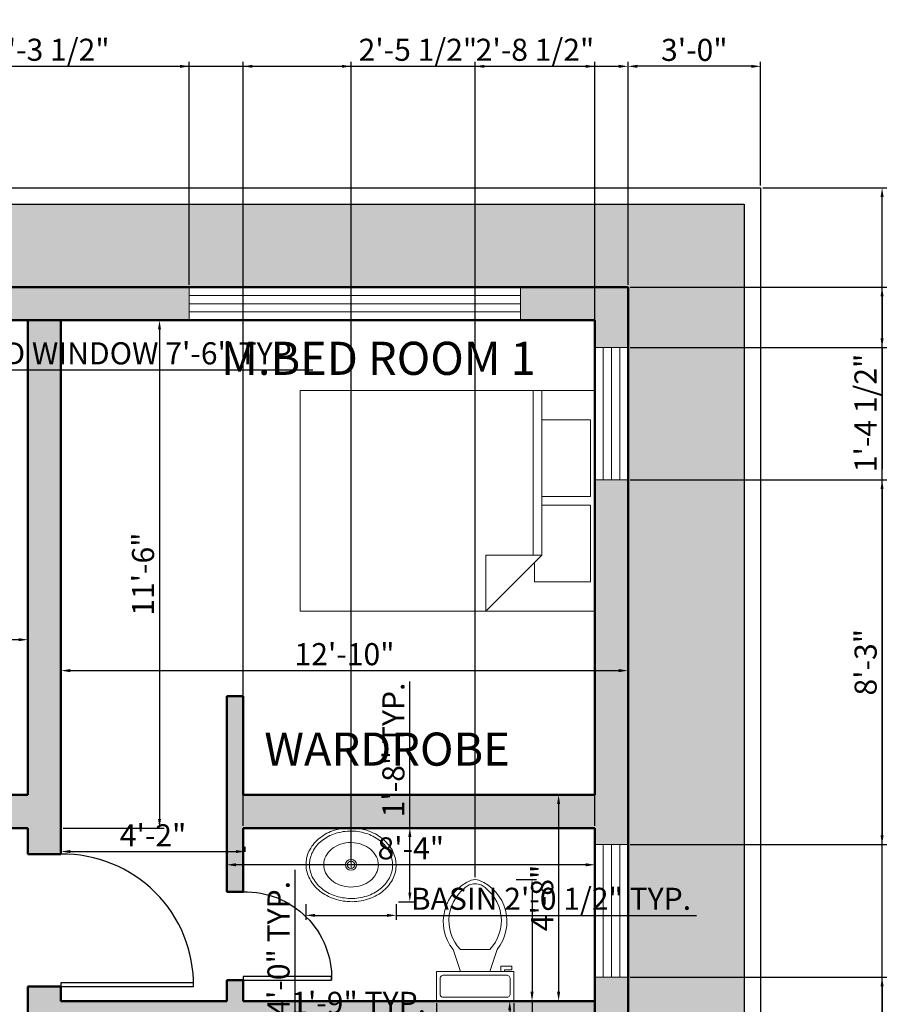
# Model space of a CAD drawing. Units: inches. Extents: x 2623 to 3157, y 1514 to 2273.
# Tile 6 of 6: x 2917 to 3157, y 1991 to 2258. Entities that reach past the tile are written whole.
import ezdxf

# ---------------------------------------------------------------- set-up
doc = ezdxf.new("R2010")
doc.units = ezdxf.units.IN
for name, color, linetype, lineweight in [('A-ANNO-DIMS', 2, 'Continuous', 18), ('A-AREA-IDEN', 7, 'Continuous', 25), ('A-DOOR', 4, 'Continuous', 25), ('A-FLOR-FIXT', 9, 'Continuous', 18), ('A-FURN', 8, 'Continuous', 18), ('A-GLAZ', 4, 'Continuous', 20), ('A-WALL', 7, 'Continuous', 50), ('A-WALL-PATT', 252, 'Continuous', 13), ('C-PROP', 7, 'Continuous', 25), ('L-PLNT-PATT', 9, 'Continuous', 13)]:
    doc.layers.add(name, color=color, linetype=linetype, lineweight=lineweight)
doc.styles.get("Standard").update_dxf_attribs({"font": 'arial.ttf'})
doc.dimstyles.new('ISO-25', dxfattribs={"dimtxt": 6, "dimasz": 2.5, "dimexe": 1.25, "dimexo": 0.625, "dimtad": 1, "dimdec": 1, "dimlunit": 3, "dimtxsty": 'Standard', "dimcen": 2.5, "dimadec": 0, "dimazin": 0, "dimtfac": 1, "dimtdec": 1, "dimtmove": 0, "dimatfit": 3, "dimfxl": 1, "dimarcsym": 0})

# ---------------------------------------------------------------- blocks, each defined once
blk = doc.blocks.new('Toilet - top')
for p, q in [((9.5, -6), (9.5, -2)), ((-8, -8.5), (-8, -8)), ((-7, -8), (-7, -9.5)), ((-4, -8), (-6, -14)), ((4, -8), (6, -14)), ((-10, -8.5), (-8, -8.5)), ((-10, -9.5), (-10, -8.5)), ((-7, -9.5), (-10, -9.5)), ((4, -14), (-4, -14))]:
    blk.add_line(p, q)
blk.add_lwpolyline([(10.5, -8), (10.5, 0), (-10.5, 0), (-10.5, -8)], close=True)
for points in [[(-9.5, -2), (-9.5, -6)], [(8.5, -1), (-8.5, -1)], [(-8.5, -7), (8.5, -7)]]:
    blk.add_lwpolyline(points)
for centre, radius, start, end in [((-8.62, -1.88), 0.884, 81.8699, 188.1301), ((8.62, -1.88), 0.884, 351.8699, 98.1301), ((-8.62, -6.12), 0.884, 171.8699, 278.1301), ((8.62, -6.12), 0.884, 261.8699, 8.1301), ((3.52, -21.58), 12.17, 141.4691, 247.9714), ((4.2, -21.82), 11.33, 136.3677, 238.9468), ((-3.52, -21.58), 12.17, 292.0284, 38.5307), ((-4.2, -21.82), 11.33, 301.053, 43.6321), ((0, -27.88), 4, 245.7318, 294.2682), ((0, -29), 4, 254.8605, 285.1395)]:
    blk.add_arc(centre, radius, start, end)
blk = doc.blocks.new('Sink - Oval top')
for p, q in [((-1, 0), (1, 0)), ((0, 1), (0, -1))]:
    blk.add_line(p, q)
for points in [[(-12.23, 0.39, 0.117634), (-11.46, -3.36, 0.104469), (-8.88, -6.8, 0.090016), (-5.08, -9.07, 0.08192), (-0.32, -10.02, 0.08192), (4.49, -9.38, 0.090016), (8.42, -7.36, 0.104469), (11.22, -4.09, 0.117634), (12.23, -0.39, 0.117634), (11.46, 3.36, 0.104469), (8.88, 6.8, 0.090016), (5.08, 9.07, 0.08192), (0.32, 10.02, 0.08192), (-4.49, 9.38, 0.090016), (-8.42, 7.36, 0.104469), (-11.22, 4.09, 0.117634)], [(-11.29, 0.16, 0.118622), (-10.52, -3.25, 0.104678), (-8.07, -6.36, 0.089562), (-4.54, -8.37, 0.081185), (-0.13, -9.15, 0.081185), (4.3, -8.49, 0.089562), (7.89, -6.58, 0.104678), (10.42, -3.55, 0.118622), (11.29, -0.16, 0.118622), (10.52, 3.25, 0.104678), (8.07, 6.36, 0.089562), (4.54, 8.37, 0.081185), (0.13, 9.15, 0.081185), (-4.3, 8.49, 0.089562), (-7.89, 6.58, 0.104678), (-10.42, 3.55, 0.118622)], [(-7.42, 0.08, 0.118283), (-6.91, -2.17, 0.104607), (-5.29, -4.21, 0.089718), (-2.97, -5.53, 0.081436), (-0.07, -6.04, 0.081436), (2.84, -5.59, 0.089718), (5.2, -4.33, 0.104607), (6.86, -2.32, 0.118283), (7.42, -0.08, 0.118283), (6.91, 2.17, 0.104607), (5.29, 4.21, 0.089718), (2.97, 5.53, 0.081436), (0.07, 6.04, 0.081436), (-2.84, 5.59, 0.089718), (-5.2, 4.33, 0.104607), (-6.86, 2.32, 0.118283)]]:
    blk.add_lwpolyline(points, format="xyb", close=True)
for radius in [1.5, 1]:
    blk.add_circle((0, 0), radius)
blk = doc.blocks.new('Window - Wood Frame 36 in. Wide plan')
for p, q in [((0, 6), (0, 0)), ((36, 6), (36, 0)), ((0, 4.5), (36, 4.5)), ((0, 3), (36, 3)), ((0, 1.5), (36, 1.5))]:
    blk.add_line(p, q)
blk = doc.blocks.new('Bed - Queen')
for p, q in [((0, -80.00003), (0, 0)), ((0, 0), (59.99999, 0)), ((59.99999, 0), (59.99999, -80.00003)), ((7.99999, -1.2), (28.79998, -1.2)), ((7.99999, -14.4), (7.99999, -1.2)), ((28.79998, -1.2), (28.79998, -14.4)), ((31.19999, -1.2), (51.99999, -1.2)), ((31.19999, -14.4), (31.19999, -1.2)), ((51.99999, -1.2), (51.99999, -16.4)), ((0, -14.4), (44.8, -14.4)), ((59.99999, -29.6), (44.8, -14.4)), ((44.8, -14.4), (44.8, -29.6)), ((44.8, -16.8), (0, -16.8)), ((51.99999, -16.4), (46.79936, -16.4)), ((44.8, -29.6), (59.99999, -29.6)), ((59.99999, -80.00003), (0, -80.00003))]:
    blk.add_line(p, q)
blk = doc.blocks.new('*D15')
at = {"layer": 'A-ANNO-DIMS', "color": 0, "lineweight": -2, "transparency": 16777216}
for p, q in [((2786.3, 2142.02), (2786.3, 2088.59)), ((2919.3, 2142.02), (2919.3, 2088.59)), ((2916.8, 2089.84), (2788.8, 2089.84))]:
    blk.add_line(p, q, dxfattribs=at)
at = {"layer": 'A-ANNO-DIMS', "color": 0, "transparency": 16777216}
for points in [[(2788.8, 2090.25), (2788.8, 2089.42), (2786.3, 2089.84)], [(2916.8, 2090.25), (2916.8, 2089.42), (2919.3, 2089.84)]]:
    blk.add_solid(points, dxfattribs=at)
at = {"layer": 'Defpoints', "color": 0, "transparency": 16777216}
for p in [(2786.3, 2142.65), (2919.3, 2142.65), (2786.3, 2089.84)]:
    blk.add_point(p, dxfattribs=at)
at = {"layer": 'A-ANNO-DIMS', "color": 0, "transparency": 16777216, "insert": (2852.8, 2093.47), "char_height": 6, "attachment_point": 5}
blk.add_mtext('11\'-1"', dxfattribs=at)
blk = doc.blocks.new('*D16')
at = {"layer": 'A-ANNO-DIMS', "color": 0, "lineweight": -2, "transparency": 16777216}
for p, q in [((2928.92, 2176.65), (2956.31, 2176.65)), ((2955.06, 2174.15), (2955.06, 2041.15)), ((2928.92, 2038.65), (2956.31, 2038.65))]:
    blk.add_line(p, q, dxfattribs=at)
at = {"layer": 'A-ANNO-DIMS', "color": 0, "transparency": 16777216}
for points in [[(2954.64, 2174.15), (2955.47, 2174.15), (2955.06, 2176.65)], [(2954.64, 2041.15), (2955.47, 2041.15), (2955.06, 2038.65)]]:
    blk.add_solid(points, dxfattribs=at)
at = {"layer": 'Defpoints', "color": 0, "transparency": 16777216}
for p in [(2928.3, 2176.65), (2928.3, 2038.65), (2955.06, 2038.65)]:
    blk.add_point(p, dxfattribs=at)
at = {"layer": 'A-ANNO-DIMS', "color": 0, "transparency": 16777216, "insert": (2951.37, 2107.65), "char_height": 6, "attachment_point": 5, "rotation": 90}
blk.add_mtext('11\'-6"', dxfattribs=at)
blk = doc.blocks.new('*D17')
at = {"layer": 'A-ANNO-DIMS', "color": 0, "lineweight": -2, "transparency": 16777216}
for p, q in [((2928.3, 2032.19), (2928.3, 2082.69)), ((3082.3, 2032.19), (3082.3, 2082.69)), ((2930.8, 2081.44), (3079.8, 2081.44))]:
    blk.add_line(p, q, dxfattribs=at)
at = {"layer": 'A-ANNO-DIMS', "color": 0, "transparency": 16777216}
for points in [[(2930.8, 2081.86), (2930.8, 2081.02), (2928.3, 2081.44)], [(3079.8, 2081.86), (3079.8, 2081.02), (3082.3, 2081.44)]]:
    blk.add_solid(points, dxfattribs=at)
at = {"layer": 'Defpoints', "color": 0, "transparency": 16777216}
for p in [(3082.3, 2081.44), (2928.3, 2031.57), (3082.3, 2031.57)]:
    blk.add_point(p, dxfattribs=at)
at = {"layer": 'A-ANNO-DIMS', "color": 0, "transparency": 16777216, "insert": (3005.3, 2085.13), "char_height": 6, "attachment_point": 5}
blk.add_mtext('12\'-10"', dxfattribs=at)
blk = doc.blocks.new('*D18')
at = {"layer": 'A-ANNO-DIMS', "color": 0, "lineweight": -2, "transparency": 16777216}
for p, q in [((2928.3, 2032.19), (2928.3, 2033.51)), ((2930.8, 2032.26), (2975.8, 2032.26)), ((2978.3, 2032.19), (2978.3, 2033.51))]:
    blk.add_line(p, q, dxfattribs=at)
at = {"layer": 'A-ANNO-DIMS', "color": 0, "transparency": 16777216}
for points in [[(2930.8, 2032.68), (2930.8, 2031.85), (2928.3, 2032.26)], [(2975.8, 2032.68), (2975.8, 2031.85), (2978.3, 2032.26)]]:
    blk.add_solid(points, dxfattribs=at)
at = {"layer": 'Defpoints', "color": 0, "transparency": 16777216}
for p in [(2928.3, 2031.57), (2978.3, 2032.26), (2978.3, 2031.57)]:
    blk.add_point(p, dxfattribs=at)
at = {"layer": 'A-ANNO-DIMS', "color": 0, "transparency": 16777216, "insert": (2953.3, 2035.9), "char_height": 6, "attachment_point": 5}
blk.add_mtext('4\'-2"', dxfattribs=at)
blk = doc.blocks.new('*D19')
at = {"layer": 'A-ANNO-DIMS', "color": 0, "lineweight": -2, "transparency": 16777216}
for p, q in [((2973.3, 2038.02), (2973.3, 2027.42)), ((3073.3, 2038.02), (3073.3, 2027.42)), ((3070.8, 2028.67), (2975.8, 2028.67))]:
    blk.add_line(p, q, dxfattribs=at)
at = {"layer": 'A-ANNO-DIMS', "color": 0, "transparency": 16777216}
for points in [[(2975.8, 2029.09), (2975.8, 2028.25), (2973.3, 2028.67)], [(3070.8, 2029.09), (3070.8, 2028.25), (3073.3, 2028.67)]]:
    blk.add_solid(points, dxfattribs=at)
at = {"layer": 'Defpoints', "color": 0, "transparency": 16777216}
for p in [(2973.3, 2038.65), (3073.3, 2038.65), (2973.3, 2028.67)]:
    blk.add_point(p, dxfattribs=at)
at = {"layer": 'A-ANNO-DIMS', "color": 0, "transparency": 16777216, "insert": (3023.3, 2032.36), "char_height": 6, "attachment_point": 5}
blk.add_mtext('8\'-4"', dxfattribs=at)
blk = doc.blocks.new('*D20')
at = {"layer": 'A-ANNO-DIMS', "color": 0, "lineweight": -2, "transparency": 16777216}
for p, q in [((3072.67, 2047.65), (3062.2, 2047.65)), ((3063.45, 2045.15), (3063.45, 1994.15)), ((3072.67, 1991.65), (3062.2, 1991.65))]:
    blk.add_line(p, q, dxfattribs=at)
at = {"layer": 'A-ANNO-DIMS', "color": 0, "transparency": 16777216}
for points in [[(3063.03, 2045.15), (3063.87, 2045.15), (3063.45, 2047.65)], [(3063.03, 1994.15), (3063.87, 1994.15), (3063.45, 1991.65)]]:
    blk.add_solid(points, dxfattribs=at)
at = {"layer": 'Defpoints', "color": 0, "transparency": 16777216}
for p in [(3073.3, 2047.65), (3063.45, 1991.65), (3073.3, 1991.65)]:
    blk.add_point(p, dxfattribs=at)
at = {"layer": 'A-ANNO-DIMS', "color": 0, "transparency": 16777216, "insert": (3059.76, 2019.65), "char_height": 6, "attachment_point": 5, "rotation": 90}
blk.add_mtext('4\'-8"', dxfattribs=at)
blk = doc.blocks.new('*D21')
at = {"layer": 'A-ANNO-DIMS', "color": 0, "lineweight": -2, "transparency": 16777216}
for p, q in [((3072.67, 1991.65), (3048.93, 1991.65)), ((3050.18, 1989.15), (3050.18, 1792.15)), ((3072.67, 1789.65), (3048.93, 1789.65))]:
    blk.add_line(p, q, dxfattribs=at)
at = {"layer": 'A-ANNO-DIMS', "color": 0, "transparency": 16777216}
for points in [[(3049.76, 1989.15), (3050.59, 1989.15), (3050.18, 1991.65)], [(3049.76, 1792.15), (3050.59, 1792.15), (3050.18, 1789.65)]]:
    blk.add_solid(points, dxfattribs=at)
at = {"layer": 'Defpoints', "color": 0, "transparency": 16777216}
for p in [(3073.3, 1991.65), (3050.18, 1789.65), (3073.3, 1789.65)]:
    blk.add_point(p, dxfattribs=at)
at = {"layer": 'A-ANNO-DIMS', "color": 0, "transparency": 16777216, "insert": (3046.49, 1890.65), "char_height": 6, "attachment_point": 5, "rotation": 90}
blk.add_mtext('16\'-10"', dxfattribs=at)
blk = doc.blocks.new('DOOR-SWING-24IN')
for p, q in [((0, 0), (0, 1)), ((0, 1), (24, 1)), ((24, 0), (0, 0)), ((24, 1), (24, 0))]:
    blk.add_line(p, q)
blk.add_arc((23.5, 0.5), 23.51, 88.7811, 181.2189)
blk = doc.blocks.new('DOOR-SWING-36IN')
for p, q in [((36, 1), (0, 1)), ((0, 1), (0, 0)), ((36, 0), (36, 1)), ((0, 0), (36, 0))]:
    blk.add_line(p, q)
blk.add_arc((0.5, 0.5), 35.5, 359.1931, 90.8069)
blk = doc.blocks.new('*D31')
at = {"layer": 'A-ANNO-DIMS', "color": 0, "lineweight": -2, "transparency": 16777216}
for p, q in [((2797.66, 2176.02), (2797.66, 2161.9)), ((2887.66, 2176.02), (2887.66, 2161.9)), ((2800.16, 2163.15), (2885.16, 2163.15)), ((2887.66, 2163.15), (2996.67, 2163.15))]:
    blk.add_line(p, q, dxfattribs=at)
at = {"layer": 'A-ANNO-DIMS', "color": 0, "transparency": 16777216}
for points in [[(2800.16, 2163.56), (2800.16, 2162.73), (2797.66, 2163.15)], [(2885.16, 2163.56), (2885.16, 2162.73), (2887.66, 2163.15)]]:
    blk.add_solid(points, dxfattribs=at)
at = {"layer": 'Defpoints', "color": 0, "transparency": 16777216}
for p in [(2797.66, 2176.65), (2887.66, 2176.65), (2887.66, 2163.15)]:
    blk.add_point(p, dxfattribs=at)
at = {"layer": 'A-ANNO-DIMS', "color": 0, "transparency": 16777216, "insert": (2943.42, 2166.88), "char_height": 6, "attachment_point": 5}
blk.add_mtext('WOOD WINDOW 7\'-6" TYP.', dxfattribs=at)
blk = doc.blocks.new('*D45')
at = {"layer": 'A-ANNO-DIMS', "color": 0, "lineweight": -2, "transparency": 16777216}
for p, q in [((2991.88, 1940.67), (2991.88, 2027.31)), ((2985.3, 1940.67), (2993.13, 1940.67)), ((2991.88, 1895.17), (2991.88, 1938.17)), ((2985.3, 1892.67), (2993.13, 1892.67))]:
    blk.add_line(p, q, dxfattribs=at)
at = {"layer": 'A-ANNO-DIMS', "color": 0, "transparency": 16777216}
for points in [[(2991.46, 1938.17), (2992.3, 1938.17), (2991.88, 1940.67)], [(2991.46, 1895.17), (2992.3, 1895.17), (2991.88, 1892.67)]]:
    blk.add_solid(points, dxfattribs=at)
at = {"layer": 'Defpoints', "color": 0, "transparency": 16777216}
for p in [(2984.68, 1940.67), (2991.88, 1940.67), (2984.68, 1892.67)]:
    blk.add_point(p, dxfattribs=at)
at = {"layer": 'A-ANNO-DIMS', "color": 0, "transparency": 16777216, "insert": (2988.15, 1985.24), "char_height": 6, "attachment_point": 5, "rotation": 90}
blk.add_mtext('LOVESEAT 4\'-0" TYP.', dxfattribs=at)
blk = doc.blocks.new('*D47')
at = {"layer": 'A-ANNO-DIMS', "color": 0, "lineweight": -2, "transparency": 16777216}
for p, q in [((3051.9, 2024.69), (3057.48, 2024.69)), ((3056.23, 2022.19), (3056.23, 1994.15)), ((3051.9, 1991.65), (3057.48, 1991.65)), ((3056.23, 1991.65), (3056.23, 1934.78))]:
    blk.add_line(p, q, dxfattribs=at)
at = {"layer": 'A-ANNO-DIMS', "color": 0, "transparency": 16777216}
for points in [[(3055.81, 2022.19), (3056.65, 2022.19), (3056.23, 2024.69)], [(3055.81, 1994.15), (3056.65, 1994.15), (3056.23, 1991.65)]]:
    blk.add_solid(points, dxfattribs=at)
at = {"layer": 'Defpoints', "color": 0, "transparency": 16777216}
for p in [(3051.27, 2024.69), (3051.27, 1991.65), (3056.23, 1991.65)]:
    blk.add_point(p, dxfattribs=at)
at = {"layer": 'A-ANNO-DIMS', "color": 0, "transparency": 16777216, "insert": (3052.5, 1961.97), "char_height": 6, "attachment_point": 5, "rotation": 90}
blk.add_mtext('WC 2\'-9" TYP.', dxfattribs=at)
blk = doc.blocks.new('*D48')
at = {"layer": 'A-ANNO-DIMS', "color": 0, "lineweight": -2, "transparency": 16777216}
for p, q in [((3030.27, 1991.02), (3030.27, 1985.44)), ((3051.27, 1991.02), (3051.27, 1985.44)), ((3030.27, 1986.69), (2990.51, 1986.69)), ((3048.77, 1986.69), (3032.77, 1986.69))]:
    blk.add_line(p, q, dxfattribs=at)
at = {"layer": 'A-ANNO-DIMS', "color": 0, "transparency": 16777216}
for points in [[(3032.77, 1987.11), (3032.77, 1986.27), (3030.27, 1986.69)], [(3048.77, 1987.11), (3048.77, 1986.27), (3051.27, 1986.69)]]:
    blk.add_solid(points, dxfattribs=at)
at = {"layer": 'Defpoints', "color": 0, "transparency": 16777216}
for p in [(3030.27, 1991.65), (3051.27, 1991.65), (3030.27, 1986.69)]:
    blk.add_point(p, dxfattribs=at)
at = {"layer": 'A-ANNO-DIMS', "color": 0, "transparency": 16777216, "insert": (3009.14, 1990.38), "char_height": 6, "attachment_point": 5}
blk.add_mtext('1\'-9" TYP.', dxfattribs=at)
blk = doc.blocks.new('*D49')
at = {"layer": 'A-ANNO-DIMS', "color": 0, "lineweight": -2, "transparency": 16777216}
for p, q in [((2994.81, 2017.98), (2994.81, 2013.67)), ((3019.36, 2017.98), (3019.36, 2013.67)), ((2997.31, 2014.92), (3016.86, 2014.92)), ((3019.36, 2014.92), (3100.88, 2014.92))]:
    blk.add_line(p, q, dxfattribs=at)
at = {"layer": 'A-ANNO-DIMS', "color": 0, "transparency": 16777216}
for points in [[(2997.31, 2015.34), (2997.31, 2014.5), (2994.81, 2014.92)], [(3016.86, 2015.34), (3016.86, 2014.5), (3019.36, 2014.92)]]:
    blk.add_solid(points, dxfattribs=at)
at = {"layer": 'Defpoints', "color": 0, "transparency": 16777216}
for p in [(2994.81, 2018.6), (3019.36, 2018.6), (3019.36, 2014.92)]:
    blk.add_point(p, dxfattribs=at)
at = {"layer": 'A-ANNO-DIMS', "color": 0, "transparency": 16777216, "insert": (3061.37, 2018.65), "char_height": 6, "attachment_point": 5}
blk.add_mtext('BASIN 2\'-0 1/2" TYP.', dxfattribs=at)
blk = doc.blocks.new('*D50')
at = {"layer": 'A-ANNO-DIMS', "color": 0, "lineweight": -2, "transparency": 16777216}
for p, q in [((3023.04, 2038.74), (3023.04, 2078.5)), ((3019.98, 2038.74), (3024.29, 2038.74)), ((3023.04, 2021.1), (3023.04, 2036.24)), ((3019.98, 2018.6), (3024.29, 2018.6))]:
    blk.add_line(p, q, dxfattribs=at)
at = {"layer": 'A-ANNO-DIMS', "color": 0, "transparency": 16777216}
for points in [[(3022.63, 2036.24), (3023.46, 2036.24), (3023.04, 2038.74)], [(3022.63, 2021.1), (3023.46, 2021.1), (3023.04, 2018.6)]]:
    blk.add_solid(points, dxfattribs=at)
at = {"layer": 'Defpoints', "color": 0, "transparency": 16777216}
for p in [(3019.36, 2038.74), (3023.04, 2038.74), (3019.36, 2018.6)]:
    blk.add_point(p, dxfattribs=at)
at = {"layer": 'A-ANNO-DIMS', "color": 0, "transparency": 16777216, "insert": (3019.35, 2059.87), "char_height": 6, "attachment_point": 5, "rotation": 90}
blk.add_mtext('1\'-8" TYP.', dxfattribs=at)
blk = doc.blocks.new('*D60')
at = {"layer": 'A-ANNO-DIMS', "color": 0, "lineweight": -2, "transparency": 16777216}
for p, q in [((3118.92, 2212.65), (3152.55, 2212.65)), ((3151.3, 1555.15), (3151.3, 2210.15)), ((3118.92, 1552.65), (3152.55, 1552.65))]:
    blk.add_line(p, q, dxfattribs=at)
at = {"layer": 'A-ANNO-DIMS', "color": 0, "transparency": 16777216}
for points in [[(3150.88, 2210.15), (3151.71, 2210.15), (3151.3, 2212.65)], [(3150.88, 1555.15), (3151.71, 1555.15), (3151.3, 1552.65)]]:
    blk.add_solid(points, dxfattribs=at)
at = {"layer": 'Defpoints', "color": 0, "transparency": 16777216}
for p in [(3118.3, 2212.65), (3151.3, 2212.65), (3118.3, 1552.65)]:
    blk.add_point(p, dxfattribs=at)
at = {"layer": 'A-ANNO-DIMS', "color": 0, "transparency": 16777216, "insert": (3147.61, 1882.65), "char_height": 6, "attachment_point": 5, "rotation": 90}
blk.add_mtext('55\'-0"', dxfattribs=at)
blk = doc.blocks.new('*D61')
at = {"layer": 'A-ANNO-DIMS', "color": 0, "lineweight": -2, "transparency": 16777216}
for p, q in [((2695.3, 2186.27), (2695.3, 2246.9)), ((2697.8, 2245.65), (3079.8, 2245.65)), ((3082.3, 2186.27), (3082.3, 2246.9))]:
    blk.add_line(p, q, dxfattribs=at)
at = {"layer": 'A-ANNO-DIMS', "color": 0, "transparency": 16777216}
for points in [[(2697.8, 2246.06), (2697.8, 2245.23), (2695.3, 2245.65)], [(3079.8, 2246.06), (3079.8, 2245.23), (3082.3, 2245.65)]]:
    blk.add_solid(points, dxfattribs=at)
at = {"layer": 'Defpoints', "color": 0, "transparency": 16777216}
for p in [(3082.3, 2245.65), (2695.3, 2185.65), (3082.3, 2185.65)]:
    blk.add_point(p, dxfattribs=at)
at = {"layer": 'A-ANNO-DIMS', "color": 0, "transparency": 16777216, "insert": (2888.8, 2249.34), "char_height": 6, "attachment_point": 5}
blk.add_mtext('32\'-3"', dxfattribs=at)
blk = doc.blocks.new('*D63')
at = {"layer": 'A-ANNO-DIMS', "color": 0, "lineweight": -2, "transparency": 16777216}
for p, q in [((3082.3, 2186.27), (3082.3, 2246.9)), ((3115.8, 2245.65), (3084.8, 2245.65)), ((3118.3, 2213.27), (3118.3, 2246.9))]:
    blk.add_line(p, q, dxfattribs=at)
at = {"layer": 'A-ANNO-DIMS', "color": 0, "transparency": 16777216}
for points in [[(3084.8, 2246.06), (3084.8, 2245.23), (3082.3, 2245.65)], [(3115.8, 2246.06), (3115.8, 2245.23), (3118.3, 2245.65)]]:
    blk.add_solid(points, dxfattribs=at)
at = {"layer": 'Defpoints', "color": 0, "transparency": 16777216}
for p in [(3082.3, 2245.65), (3118.3, 2212.65), (3082.3, 2185.65)]:
    blk.add_point(p, dxfattribs=at)
at = {"layer": 'A-ANNO-DIMS', "color": 0, "transparency": 16777216, "insert": (3100.3, 2249.34), "char_height": 6, "attachment_point": 5}
blk.add_mtext('3\'-0"', dxfattribs=at)
blk = doc.blocks.new('*D78')
at = {"layer": 'A-ANNO-DIMS', "color": 0, "lineweight": -2, "transparency": 16777216}
for p, q in [((2887.66, 2186.27), (2887.66, 2246.9)), ((2890.16, 2245.65), (2960.63, 2245.65)), ((2963.13, 2186.27), (2963.13, 2246.9))]:
    blk.add_line(p, q, dxfattribs=at)
at = {"layer": 'A-ANNO-DIMS', "color": 0, "transparency": 16777216}
for points in [[(2890.16, 2246.06), (2890.16, 2245.23), (2887.66, 2245.65)], [(2960.63, 2246.06), (2960.63, 2245.23), (2963.13, 2245.65)]]:
    blk.add_solid(points, dxfattribs=at)
at = {"layer": 'Defpoints', "color": 0, "transparency": 16777216}
for p in [(2963.13, 2245.65), (2887.66, 2185.65), (2963.13, 2185.65)]:
    blk.add_point(p, dxfattribs=at)
at = {"layer": 'A-ANNO-DIMS', "color": 0, "transparency": 16777216, "insert": (2925.4, 2249.38), "char_height": 6, "attachment_point": 5}
blk.add_mtext('6\'-3 1/2"', dxfattribs=at)
blk = doc.blocks.new('*D86')
at = {"layer": 'A-ANNO-DIMS', "color": 0, "lineweight": -2, "transparency": 16777216}
for p, q in [((2977.8, 2039.27), (2977.8, 2246.9)), ((2980.3, 2245.65), (3004.58, 2245.65)), ((3007.08, 2029.29), (3007.08, 2246.9)), ((3007.08, 2245.65), (3040.87, 2245.65))]:
    blk.add_line(p, q, dxfattribs=at)
at = {"layer": 'A-ANNO-DIMS', "color": 0, "transparency": 16777216}
for points in [[(2980.3, 2246.06), (2980.3, 2245.23), (2977.8, 2245.65)], [(3004.58, 2246.06), (3004.58, 2245.23), (3007.08, 2245.65)]]:
    blk.add_solid(points, dxfattribs=at)
at = {"layer": 'Defpoints', "color": 0, "transparency": 16777216}
for p in [(3007.08, 2245.65), (2977.8, 2038.65), (3007.08, 2028.67)]:
    blk.add_point(p, dxfattribs=at)
at = {"layer": 'A-ANNO-DIMS', "color": 0, "transparency": 16777216, "insert": (3025.23, 2249.37), "char_height": 6, "attachment_point": 5}
blk.add_mtext('2\'-5 1/2"', dxfattribs=at)
blk = doc.blocks.new('*D87')
at = {"layer": 'A-ANNO-DIMS', "color": 0, "lineweight": -2, "transparency": 16777216}
for p, q in [((3040.77, 2025.27), (3040.77, 2246.9)), ((3043.27, 2245.65), (3070.8, 2245.65)), ((3073.3, 2039.27), (3073.3, 2246.9))]:
    blk.add_line(p, q, dxfattribs=at)
at = {"layer": 'A-ANNO-DIMS', "color": 0, "transparency": 16777216}
for points in [[(3043.27, 2246.06), (3043.27, 2245.23), (3040.77, 2245.65)], [(3070.8, 2246.06), (3070.8, 2245.23), (3073.3, 2245.65)]]:
    blk.add_solid(points, dxfattribs=at)
at = {"layer": 'Defpoints', "color": 0, "transparency": 16777216}
for p in [(3073.3, 2245.65), (3073.3, 2038.65), (3040.77, 2024.65)]:
    blk.add_point(p, dxfattribs=at)
at = {"layer": 'A-ANNO-DIMS', "color": 0, "transparency": 16777216, "insert": (3057.03, 2249.37), "char_height": 6, "attachment_point": 5}
blk.add_mtext('2\'-8 1/2"', dxfattribs=at)
blk = doc.blocks.new('*D92')
at = {"layer": 'A-ANNO-DIMS', "color": 0, "lineweight": -2, "transparency": 16777216}
for p, q in [((3082.92, 2185.65), (3152.55, 2185.65)), ((3151.3, 2183.15), (3151.3, 2171.76)), ((3082.92, 2169.26), (3152.55, 2169.26)), ((3151.3, 2169.26), (3151.3, 2136.15))]:
    blk.add_line(p, q, dxfattribs=at)
at = {"layer": 'A-ANNO-DIMS', "color": 0, "transparency": 16777216}
for points in [[(3150.88, 2183.15), (3151.71, 2183.15), (3151.3, 2185.65)], [(3150.88, 2171.76), (3151.71, 2171.76), (3151.3, 2169.26)]]:
    blk.add_solid(points, dxfattribs=at)
at = {"layer": 'Defpoints', "color": 0, "transparency": 16777216}
for p in [(3082.3, 2185.65), (3082.3, 2169.26), (3151.3, 2169.26)]:
    blk.add_point(p, dxfattribs=at)
at = {"layer": 'A-ANNO-DIMS', "color": 0, "transparency": 16777216, "insert": (3147.57, 2151.45), "char_height": 6, "attachment_point": 5, "rotation": 90}
blk.add_mtext('1\'-4 1/2"', dxfattribs=at)
blk = doc.blocks.new('*D93')
at = {"layer": 'A-ANNO-DIMS', "color": 0, "lineweight": -2, "transparency": 16777216}
for p, q in [((3082.92, 2133.26), (3152.55, 2133.26)), ((3151.3, 2130.76), (3151.3, 2036.66)), ((3082.92, 2034.16), (3152.55, 2034.16))]:
    blk.add_line(p, q, dxfattribs=at)
at = {"layer": 'A-ANNO-DIMS', "color": 0, "transparency": 16777216}
for points in [[(3150.88, 2130.76), (3151.71, 2130.76), (3151.3, 2133.26)], [(3150.88, 2036.66), (3151.71, 2036.66), (3151.3, 2034.16)]]:
    blk.add_solid(points, dxfattribs=at)
at = {"layer": 'Defpoints', "color": 0, "transparency": 16777216}
for p in [(3082.3, 2133.26), (3082.3, 2034.16), (3151.3, 2034.16)]:
    blk.add_point(p, dxfattribs=at)
at = {"layer": 'A-ANNO-DIMS', "color": 0, "transparency": 16777216, "insert": (3147.61, 2083.71), "char_height": 6, "attachment_point": 5, "rotation": 90}
blk.add_mtext('8\'-3"', dxfattribs=at)
blk = doc.blocks.new('*D94')
at = {"layer": 'A-ANNO-DIMS', "color": 0, "lineweight": -2, "transparency": 16777216}
for p, q in [((3082.92, 1998.16), (3152.55, 1998.16)), ((3151.3, 1995.66), (3151.3, 1977.07)), ((3082.92, 1974.57), (3152.55, 1974.57)), ((3151.3, 1974.57), (3151.3, 1936.8))]:
    blk.add_line(p, q, dxfattribs=at)
at = {"layer": 'A-ANNO-DIMS', "color": 0, "transparency": 16777216}
for points in [[(3150.88, 1995.66), (3151.71, 1995.66), (3151.3, 1998.16)], [(3150.88, 1977.07), (3151.71, 1977.07), (3151.3, 1974.57)]]:
    blk.add_solid(points, dxfattribs=at)
at = {"layer": 'Defpoints', "color": 0, "transparency": 16777216}
for p in [(3082.3, 1998.16), (3082.3, 1974.57), (3151.3, 1974.57)]:
    blk.add_point(p, dxfattribs=at)
at = {"layer": 'A-ANNO-DIMS', "color": 0, "transparency": 16777216, "insert": (3147.57, 1954.44), "char_height": 6, "attachment_point": 5, "rotation": 90}
blk.add_mtext('1\'-11 1/2"', dxfattribs=at)

msp = doc.modelspace()

# ---------------------------------------------------------------- hatches: boundary and pattern name
at = {"layer": 'A-WALL-PATT'}
h = msp.add_hatch(color=256, dxfattribs=at)
h.dxf.hatch_style = 1
h.paths.add_polyline_path([(2704.3, 1854.65), (2893.38, 1854.65), (2893.38, 1850.02), (2902.38, 1850.02), (2902.38, 1863.65), (2704.3, 1863.65), (2704.3, 1949.25), (2695.3, 1949.25), (2695.3, 1845.57), (2704.3, 1845.57)])
h.paths.add_polyline_path([(2704.3, 1809.57), (2695.3, 1809.57), (2695.3, 1750.74), (2704.3, 1750.74)])
h.paths.add_polyline_path([(2764.7, 1621.65), (2704.3, 1621.65), (2704.3, 1660.74), (2695.3, 1660.74), (2695.3, 1612.65), (2764.7, 1612.65)])
h.paths.add_polyline_path([(2704.3, 2128.1), (2695.3, 2128.1), (2695.3, 2039.25), (2704.3, 2039.25)])
h.paths.add_polyline_path([(2714, 2185.65), (2695.3, 2185.65), (2695.3, 2164.1), (2704.3, 2164.1), (2704.3, 2176.65), (2714, 2176.65)])
h.paths.add_polyline_path([(2797.66, 2185.65), (2768, 2185.65), (2768, 2176.65), (2797.66, 2176.65)])
h.paths.add_polyline_path([(2777.8, 2176.65), (2773.3, 2176.65), (2773.3, 2142.65), (2777.8, 2142.65)])
h.paths.add_polyline_path([(2963.13, 2185.65), (2887.66, 2185.65), (2887.66, 2176.65), (2963.13, 2176.65)])
h.paths.add_polyline_path([(2928.3, 2176.65), (2919.3, 2176.65), (2919.3, 2047.65), (2850.8, 2047.65), (2850.8, 2038.65), (2919.3, 2038.65), (2919.3, 2031.57), (2928.3, 2031.57), (2928.3, 2038.65)])
h.paths.add_polyline_path([(3082.3, 2185.65), (3053.13, 2185.65), (3053.13, 2176.65), (3073.3, 2176.65), (3073.3, 2169.26), (3082.3, 2169.26)])
h.paths.add_polyline_path([(3082.3, 2133.26), (3073.3, 2133.26), (3073.3, 2047.65), (2977.8, 2047.65), (2977.8, 2074.51), (2973.3, 2074.51), (2973.3, 2047.65), (2973.3, 2038.65), (2973.3, 2021.33), (2977.8, 2021.33), (2977.8, 2038.65), (3005.74, 2038.65, -0.027912), (3007.41, 2038.69, -0.0118), (3008.11, 2038.65), (3073.3, 2038.65), (3073.3, 2034.16), (3082.3, 2034.16)])
h.paths.add_polyline_path([(3082.3, 1998.16), (3073.3, 1998.16), (3073.3, 1991.65), (2977.8, 1991.65), (2977.8, 1997.33), (2973.3, 1997.33), (2973.3, 1991.65), (2928.3, 1991.65), (2928.3, 1995.57), (2919.3, 1995.57), (2919.3, 1982.65), (3073.3, 1982.65), (3073.3, 1974.57), (3082.3, 1974.57)])
at = {"layer": 'L-PLNT-PATT'}
h = msp.add_hatch(color=256, dxfattribs=at)
h.dxf.hatch_style = 1
h.set_gradient(color1=(19, 155, 72), color2=(63, 255, 0), name='CURVED')
h.paths.add_polyline_path([(2902.38, 1612.65), (2695.3, 1612.65), (2695.3, 2185.65), (3082.3, 2185.65), (3082.3, 1780.65), (3113.8, 1780.65), (3113.8, 2208.15), (2672.8, 2208.15), (2672.8, 1557.15), (2902.38, 1557.15)])
h = msp.add_hatch(color=256, dxfattribs=at)
h.dxf.hatch_style = 1
h.set_gradient(color1=(19, 155, 72), color2=(63, 255, 0), name='CYLINDER')
h.paths.add_polyline_path([(3024.32, 1726.09), (2994.86, 1726.09), (2994.86, 1587.38), (3024.32, 1587.38)], flags=17)
h.paths.add_polyline_path([(2902.38, 1612.65), (2695.3, 1612.65), (2695.3, 2185.65), (3082.3, 2185.65), (3082.3, 1780.65), (3113.8, 1780.65), (3113.8, 2208.15), (2672.8, 2208.15), (2672.8, 1557.15), (2902.38, 1557.15)])

# ---------------------------------------------------------------- linework, layer by layer
at = {"layer": 'A-GLAZ'}
for p, q in [((2963.13, 2185.65), (2963.13, 2176.65)), ((3053.13, 2185.65), (3053.13, 2176.65)), ((3073.3, 2169.26), (3082.3, 2169.26)), ((3073.3, 2133.26), (3082.3, 2133.26)), ((3073.3, 2034.16), (3082.3, 2034.16)), ((3073.3, 1998.16), (3082.3, 1998.16))]:
    msp.add_line(p, q, dxfattribs=at)
at = {"layer": 'A-WALL'}
for p, q in [((2695.3, 2185.65), (3082.3, 2185.65)), ((3082.3, 2185.65), (3082.3, 1780.65)), ((2704.3, 2176.65), (3073.3, 2176.65)), ((2919.3, 2176.65), (2919.3, 2047.65)), ((2928.3, 2176.65), (2928.3, 2038.65)), ((3073.3, 2176.65), (3073.3, 2047.65)), ((2973.3, 2047.65), (2973.3, 2074.51)), ((2973.3, 2074.51), (2977.8, 2074.51)), ((2977.8, 2074.51), (2977.8, 2047.65)), ((2850.8, 2047.65), (2919.3, 2047.65)), ((2973.3, 2038.65), (2973.3, 2047.65)), ((2977.8, 2047.65), (3073.3, 2047.65)), ((2977.8, 2047.65), (3073.3, 2047.65)), ((2850.8, 2038.65), (2919.3, 2038.65)), ((2919.3, 2031.57), (2919.3, 2038.65)), ((2928.3, 2031.57), (2928.3, 2038.65)), ((2973.3, 2038.65), (2973.3, 2021.33)), ((2977.8, 2038.65), (3073.3, 2038.65)), ((2977.8, 2038.65), (2977.8, 2021.33)), ((2977.8, 2038.65), (3073.3, 2038.65)), ((3073.3, 2038.65), (3073.3, 1991.65)), ((2928.3, 2031.57), (2919.3, 2031.57)), ((2977.8, 2021.33), (2973.3, 2021.33)), ((2973.3, 1997.33), (2977.8, 1997.33)), ((2973.3, 1997.33), (2973.3, 1991.65)), ((2977.8, 1991.65), (2977.8, 1997.33)), ((2977.8, 1997.33), (2977.8, 1991.65)), ((2919.3, 1982.65), (2919.3, 1995.57)), ((2919.3, 1995.57), (2928.3, 1995.57)), ((2928.3, 1991.65), (2928.3, 1995.57)), ((2928.3, 1991.65), (2973.3, 1991.65)), ((2977.8, 1991.65), (3073.3, 1991.65)), ((3073.3, 1991.65), (3073.3, 1789.65))]:
    msp.add_line(p, q, dxfattribs=at)
at = {"layer": 'C-PROP'}
for p, q in [((2668.3, 2212.65), (3118.3, 2212.65)), ((3118.3, 2212.65), (3118.3, 1552.65)), ((2672.8, 2208.15), (3113.8, 2208.15)), ((3113.8, 2208.15), (3113.8, 1557.15))]:
    msp.add_line(p, q, dxfattribs=at)

# ---------------------------------------------------------------- block references
at = {"layer": 'A-DOOR'}
msp.add_blockref('DOOR-SWING-36IN', (2928.3, 1995.57), dxfattribs=at)
at = {"layer": 'A-DOOR', "extrusion": (0, 0, -1), "zscale": -1}
msp.add_blockref('DOOR-SWING-24IN', (-3001.8, 1997.33), dxfattribs=at)
at = {"layer": 'A-FLOR-FIXT'}
msp.add_blockref('Sink - Oval top', (3007.08, 2028.67), dxfattribs=at)
at = {"layer": 'A-FLOR-FIXT', "rotation": 180}
msp.add_blockref('Toilet - top', (3040.77, 1991.65), dxfattribs=at)
at = {"layer": 'A-FURN', "rotation": 270}
msp.add_blockref('Bed - Queen', (3073.3, 2157.57), dxfattribs=at)
at = {"layer": 'A-GLAZ', "xscale": 2.5, "yscale": 1.5}
msp.add_blockref('Window - Wood Frame 36 in. Wide plan', (2963.13, 2176.65), dxfattribs=at)
at = {"layer": 'A-GLAZ', "yscale": 1.5, "rotation": 90}
for p in [(3082.3, 2133.26), (3082.3, 1998.16)]:
    msp.add_blockref('Window - Wood Frame 36 in. Wide plan', p, dxfattribs=at)

# ---------------------------------------------------------------- texts
at = {"layer": 'A-AREA-IDEN', "char_height": 9, "attachment_point": 1}
for s, insert in [('M.BED ROOM 1', (2971.81, 2170.8)), ('WARDROBE', (2983.51, 2064.6))]:
    msp.add_mtext(s, dxfattribs=dict(at, insert=insert))

# ---------------------------------------------------------------- dimensions: what is measured, and where the dimension line sits
at = {"layer": 'A-ANNO-DIMS'}
for base, p1, p2, override, picture, middle in [((2963.13, 2245.65), (2887.66, 2185.65), (2963.13, 2185.65), {"dimdec": 1, "dimlfac": 1, "dimrnd": 0, "dimzin": 1, "dimdsep": 46, "dimlunit": 4, "dimfrac": 2}, '*D78', (2925.4, 2249.38)), ((3007.08, 2245.65), (2977.8, 2038.65), (3007.08, 2028.67), {"dimdec": 1, "dimlfac": 1, "dimrnd": 0, "dimzin": 1, "dimdsep": 46, "dimlunit": 4, "dimfrac": 2}, '*D86', (3025.23, 2249.37)), ((3073.3, 2245.65), (3040.77, 2024.65), (3073.3, 2038.65), {"dimdec": 1, "dimlfac": 1, "dimrnd": 0, "dimzin": 1, "dimdsep": 46, "dimlunit": 4, "dimfrac": 2}, '*D87', (3057.03, 2249.37)), ((3082.3, 2245.65), (2695.3, 2185.65), (3082.3, 2185.65), {"dimdec": 1, "dimlfac": 1, "dimrnd": 0, "dimzin": 1, "dimdsep": 46, "dimlunit": 4, "dimfrac": 2}, '*D61', (2888.8, 2249.34)), ((3082.3, 2245.65), (3118.3, 2212.65), (3082.3, 2185.65), {"dimdec": 1, "dimlfac": 1, "dimrnd": 0, "dimzin": 1, "dimdsep": 46, "dimlunit": 4, "dimfrac": 2}, '*D63', (3100.3, 2249.34)), ((2786.3, 2089.84), (2919.3, 2142.65), (2786.3, 2142.65), {"dimclrd": 0, "dimclre": 0, "dimclrt": 0}, '*D15', (2852.8, 2093.47)), ((3082.3, 2081.44), (2928.3, 2031.57), (3082.3, 2031.57), {"dimclrd": 0, "dimclre": 0, "dimclrt": 0}, '*D17', (3005.3, 2085.13)), ((2978.3, 2032.26), (2928.3, 2031.57), (2978.3, 2031.57), {"dimclrd": 0, "dimclre": 0, "dimclrt": 0}, '*D18', (2953.3, 2035.9)), ((2973.3, 2028.67), (3073.3, 2038.65), (2973.3, 2038.65), {"dimclrd": 0, "dimclre": 0, "dimclrt": 0}, '*D19', (3023.3, 2032.36))]:
    dim = msp.add_linear_dim(base=base, p1=p1, p2=p2, dimstyle='ISO-25', override=override, dxfattribs=at)
    dim.commit()
    dim.dimension.update_dxf_attribs({"geometry": picture, "text_midpoint": middle})
for base, p1, p2, override, picture, middle in [((3151.3, 2212.65), (3118.3, 1552.65), (3118.3, 2212.65), {"dimdec": 1, "dimlfac": 1, "dimrnd": 0, "dimzin": 1, "dimdsep": 46, "dimlunit": 4, "dimfrac": 2}, '*D60', (3147.61, 1882.65)), ((3151.3, 2169.26), (3082.3, 2185.65), (3082.3, 2169.26), {"dimdec": 1, "dimlfac": 1, "dimrnd": 0, "dimzin": 1, "dimdsep": 46, "dimlunit": 4, "dimfrac": 2}, '*D92', (3147.57, 2151.45)), ((2955.06, 2038.65), (2928.3, 2176.65), (2928.3, 2038.65), {"dimclrd": 0, "dimclre": 0, "dimclrt": 0}, '*D16', (2951.37, 2107.65)), ((3151.3, 2034.16), (3082.3, 2133.26), (3082.3, 2034.16), {"dimdec": 1, "dimlfac": 1, "dimrnd": 0, "dimzin": 1, "dimdsep": 46, "dimlunit": 4, "dimfrac": 2}, '*D93', (3147.61, 2083.71)), ((3063.45, 1991.65), (3073.3, 2047.65), (3073.3, 1991.65), {"dimclrd": 0, "dimclre": 0, "dimclrt": 0}, '*D20', (3059.76, 2019.65)), ((3151.3, 1974.57), (3082.3, 1998.16), (3082.3, 1974.57), {"dimdec": 1, "dimlfac": 1, "dimrnd": 0, "dimzin": 1, "dimdsep": 46, "dimlunit": 4, "dimfrac": 2}, '*D94', (3147.57, 1954.44)), ((3050.18, 1789.65), (3073.3, 1991.65), (3073.3, 1789.65), {"dimclrd": 0, "dimclre": 0, "dimclrt": 0}, '*D21', (3046.49, 1890.65))]:
    dim = msp.add_linear_dim(base=base, p1=p1, p2=p2, angle=90, dimstyle='ISO-25', override=override, dxfattribs=at)
    dim.commit()
    dim.dimension.update_dxf_attribs({"geometry": picture, "text_midpoint": middle})
for base, p1, p2, text, picture, middle in [((2887.66, 2163.15), (2797.66, 2176.65), (2887.66, 2176.65), 'WOOD WINDOW <> TYP.', '*D31', (2943.42, 2166.88)), ((3019.3599, 2014.9189), (2994.809, 2018.6015), (3019.3599, 2018.6015), 'BASIN <> TYP.', '*D49', (3061.3703, 2018.6462))]:
    dim = msp.add_linear_dim(base=base, p1=p1, p2=p2, text=text, dimstyle='ISO-25', override={"dimdec": 1, "dimlfac": 1, "dimrnd": 0, "dimzin": 1, "dimdsep": 46, "dimlunit": 4, "dimfrac": 2}, dxfattribs=at)
    dim.commit()
    dim.dimension.update_dxf_attribs({"geometry": picture, "text_midpoint": middle})
for base, p1, p2, angle, text, picture, middle in [((3023.04, 2038.74), (3019.36, 2018.6), (3019.36, 2038.74), 90, '<> TYP.', '*D50', (3019.35, 2059.87)), ((2991.88, 1940.67), (2984.68, 1892.67), (2984.68, 1940.67), 90, 'LOVESEAT <> TYP.', '*D45', (2988.15, 1985.24)), ((3056.23, 1991.65), (3051.27, 2024.69), (3051.27, 1991.65), 270, 'WC <> TYP.', '*D47', (3052.5, 1961.97)), ((3030.27, 1986.69), (3051.27, 1991.65), (3030.27, 1991.65), 180, '<> TYP.', '*D48', (3009.14, 1990.38))]:
    dim = msp.add_linear_dim(base=base, p1=p1, p2=p2, angle=angle, text=text, dimstyle='ISO-25', override={"dimdec": 1, "dimlfac": 1, "dimrnd": 0, "dimzin": 1, "dimdsep": 46, "dimlunit": 4, "dimfrac": 2}, dxfattribs=at)
    dim.commit()
    dim.dimension.update_dxf_attribs({"geometry": picture, "text_midpoint": middle})

doc.saveas('drawing.dxf')
